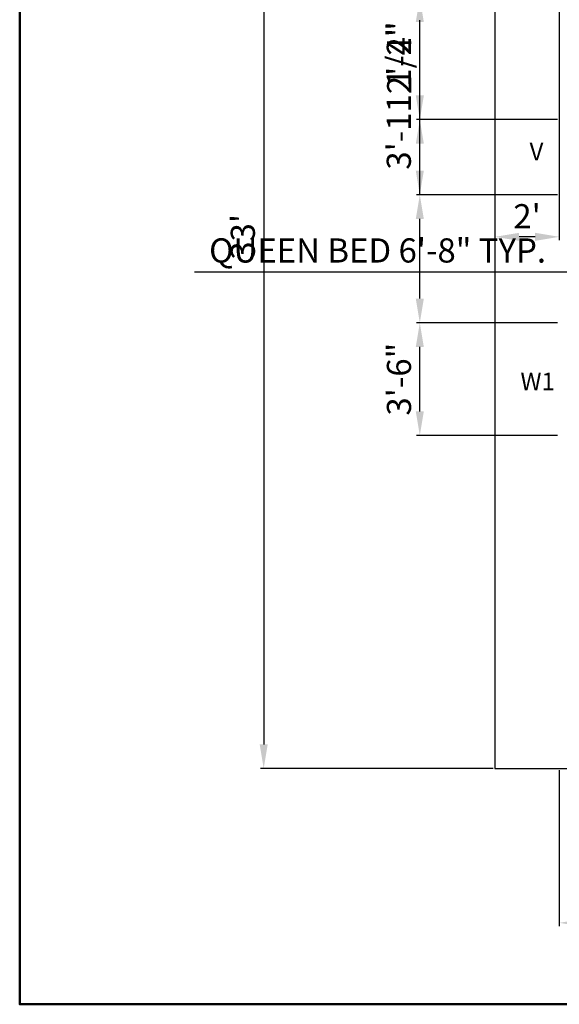
# Model space of a CAD drawing. Units: inches. Extents: x 2113 to 4530, y 1685 to 2353.
# Tile 1 of 6: x 2113 to 2314, y 1685 to 2052. Entities that reach past the tile are written whole.
import ezdxf

# ---------------------------------------------------------------- set-up
doc = ezdxf.new("R2010")
doc.units = ezdxf.units.IN
for name, color, linetype, lineweight in [('A-ANNO-DIMS', 2, 'Continuous', 18), ('A-ANNO-TEXT', 7, 'Continuous', 18), ('A-ANNO-TTLB', 7, 'Continuous', 50), ('C-PROP', 7, 'Continuous', 25), ('S-ANNO-DIMS', 2, 'Continuous', 18)]:
    doc.layers.add(name, color=color, linetype=linetype, lineweight=lineweight)
doc.styles.get("Standard").update_dxf_attribs({"font": 'arial.ttf'})
doc.dimstyles.new('ISO-25', dxfattribs={"dimtxt": 9, "dimasz": 9, "dimexe": 1.25, "dimexo": 0.625, "dimgap": 2, "dimtad": 1, "dimdec": 1, "dimlunit": 4, "dimtxsty": 'Standard', "dimcen": 2.5, "dimazin": 0, "dimtfac": 1, "dimtdec": 1, "dimtmove": 0, "dimatfit": 3, "dimfxl": 1, "dimarcsym": 0})

# ---------------------------------------------------------------- blocks, each defined once
blk = doc.blocks.new('*D8')
at = {"layer": 'A-ANNO-DIMS', "color": 0, "lineweight": -2, "transparency": 16777216}
for p, q in [((2289.11, 2168.89), (2202.39, 2168.89)), ((2203.64, 2159.89), (2203.64, 1781.89)), ((2289.11, 1772.89), (2202.39, 1772.89))]:
    blk.add_line(p, q, dxfattribs=at)
at = {"layer": 'A-ANNO-DIMS', "color": 0, "transparency": 16777216}
for points in [[(2202.14, 2159.89), (2205.14, 2159.89), (2203.64, 2168.89)], [(2202.14, 1781.89), (2205.14, 1781.89), (2203.64, 1772.89)]]:
    blk.add_solid(points, dxfattribs=at)
at = {"layer": 'Defpoints', "color": 0, "transparency": 16777216}
for p in [(2289.73, 2168.89), (2203.64, 1772.89), (2289.73, 1772.89)]:
    blk.add_point(p, dxfattribs=at)
at = {"layer": 'A-ANNO-DIMS', "color": 0, "transparency": 16777216, "insert": (2197.04, 1970.89), "char_height": 9, "attachment_point": 5, "rotation": 90}
blk.add_mtext("33'", dxfattribs=at)
blk = doc.blocks.new('*D29')
at = {"layer": 'A-ANNO-DIMS', "color": 0, "lineweight": -2, "transparency": 16777216}
for p, q in [((2289.73, 2168.26), (2289.73, 1969.64)), ((2313.73, 2150.26), (2313.73, 1969.64)), ((2304.73, 1970.89), (2298.73, 1970.89))]:
    blk.add_line(p, q, dxfattribs=at)
at = {"layer": 'A-ANNO-DIMS', "color": 0, "transparency": 16777216}
for points in [[(2298.73, 1972.39), (2298.73, 1969.39), (2289.73, 1970.89)], [(2304.73, 1972.39), (2304.73, 1969.39), (2313.73, 1970.89)]]:
    blk.add_solid(points, dxfattribs=at)
at = {"layer": 'Defpoints', "color": 0, "transparency": 16777216}
for p in [(2289.73, 2168.89), (2313.73, 2150.89), (2289.73, 1970.89)]:
    blk.add_point(p, dxfattribs=at)
at = {"layer": 'A-ANNO-DIMS', "color": 0, "transparency": 16777216, "insert": (2301.73, 1977.4), "char_height": 9, "attachment_point": 5}
blk.add_mtext("2'", dxfattribs=at)
blk = doc.blocks.new('LOT-465X396')
for p, q in [((0, 396), (0, 0)), ((0, 0), (465, 0))]:
    blk.add_line(p, q)
blk = doc.blocks.new('*D40')
at = {"layer": 'Defpoints', "color": 0, "transparency": 16777216}
for p in [(2323.25, 1957.72), (2323.25, 1945.72), (2403.25, 1945.72)]:
    blk.add_point(p, dxfattribs=at)
at = {"layer": 'S-ANNO-DIMS', "color": 0, "lineweight": -2, "transparency": 16777216}
for p, q in [((2323.25, 1946.35), (2323.25, 1958.97)), ((2403.25, 1946.35), (2403.25, 1958.97)), ((2323.25, 1957.72), (2177.86, 1957.72)), ((2394.25, 1957.72), (2332.25, 1957.72))]:
    blk.add_line(p, q, dxfattribs=at)
at = {"layer": 'S-ANNO-DIMS', "color": 0, "transparency": 16777216}
for points in [[(2332.25, 1959.22), (2332.25, 1956.22), (2323.25, 1957.72)], [(2394.25, 1959.22), (2394.25, 1956.22), (2403.25, 1957.72)]]:
    blk.add_solid(points, dxfattribs=at)
at = {"layer": 'S-ANNO-DIMS', "color": 0, "transparency": 16777216, "insert": (2246.05, 1964.65), "char_height": 9, "attachment_point": 5}
blk.add_mtext('QUEEN BED 6\'-8" TYP.', dxfattribs=at)
blk = doc.blocks.new('*D90')
at = {"layer": 'Defpoints', "color": 0, "transparency": 16777216}
for p in [(2313.73, 1772.89), (2456.73, 1772.89), (2456.73, 1715.45)]:
    blk.add_point(p, dxfattribs=at)
at = {"layer": 'S-ANNO-DIMS', "color": 0, "lineweight": -2, "transparency": 16777216}
for p, q in [((2313.73, 1772.26), (2313.73, 1714.2)), ((2456.73, 1772.26), (2456.73, 1714.2)), ((2322.73, 1715.45), (2447.73, 1715.45))]:
    blk.add_line(p, q, dxfattribs=at)
at = {"layer": 'S-ANNO-DIMS', "color": 0, "transparency": 16777216}
for points in [[(2322.73, 1716.95), (2322.73, 1713.95), (2313.73, 1715.45)], [(2447.73, 1716.95), (2447.73, 1713.95), (2456.73, 1715.45)]]:
    blk.add_solid(points, dxfattribs=at)
at = {"layer": 'S-ANNO-DIMS', "color": 0, "transparency": 16777216, "insert": (2385.23, 1721.97), "char_height": 9, "attachment_point": 5}
blk.add_mtext('11\'-11"', dxfattribs=at)
blk = doc.blocks.new('*D95')
at = {"layer": 'Defpoints', "color": 0, "transparency": 16777216}
for p in [(2261.78, 1938.89), (2313.73, 1938.89), (2313.73, 1896.89)]:
    blk.add_point(p, dxfattribs=at)
at = {"layer": 'S-ANNO-DIMS', "color": 0, "lineweight": -2, "transparency": 16777216}
for p, q in [((2313.11, 1938.89), (2260.53, 1938.89)), ((2261.78, 1905.89), (2261.78, 1929.89)), ((2313.11, 1896.89), (2260.53, 1896.89))]:
    blk.add_line(p, q, dxfattribs=at)
at = {"layer": 'S-ANNO-DIMS', "color": 0, "transparency": 16777216}
for points in [[(2260.28, 1929.89), (2263.28, 1929.89), (2261.78, 1938.89)], [(2260.28, 1905.89), (2263.28, 1905.89), (2261.78, 1896.89)]]:
    blk.add_solid(points, dxfattribs=at)
at = {"layer": 'S-ANNO-DIMS', "color": 0, "transparency": 16777216, "insert": (2255.18, 1917.89), "char_height": 9, "attachment_point": 5, "rotation": 90}
blk.add_mtext('3\'-6"', dxfattribs=at)
blk = doc.blocks.new('*D96')
at = {"layer": 'Defpoints', "color": 0, "transparency": 16777216}
for p in [(2261.78, 1986.53), (2313.73, 1986.53), (2313.73, 1938.89)]:
    blk.add_point(p, dxfattribs=at)
at = {"layer": 'S-ANNO-DIMS', "color": 0, "lineweight": -2, "transparency": 16777216}
for p, q in [((2261.78, 1986.53), (2261.78, 2051.42)), ((2313.11, 1986.53), (2260.53, 1986.53)), ((2261.78, 1947.89), (2261.78, 1977.53)), ((2313.11, 1938.89), (2260.53, 1938.89))]:
    blk.add_line(p, q, dxfattribs=at)
at = {"layer": 'S-ANNO-DIMS', "color": 0, "transparency": 16777216}
for points in [[(2260.28, 1977.53), (2263.28, 1977.53), (2261.78, 1986.53)], [(2260.28, 1947.89), (2263.28, 1947.89), (2261.78, 1938.89)]]:
    blk.add_solid(points, dxfattribs=at)
at = {"layer": 'S-ANNO-DIMS', "color": 0, "transparency": 16777216, "insert": (2255.13, 2023.47), "char_height": 9, "attachment_point": 5, "rotation": 90}
blk.add_mtext('3\'-11 1/2"', dxfattribs=at)
blk = doc.blocks.new('*D97')
at = {"layer": 'Defpoints', "color": 0, "transparency": 16777216}
for p in [(2261.78, 2014.53), (2313.73, 2014.53), (2313.73, 1986.53)]:
    blk.add_point(p, dxfattribs=at)
at = {"layer": 'S-ANNO-DIMS', "color": 0, "lineweight": -2, "transparency": 16777216}
for p, q in [((2261.78, 2014.53), (2261.78, 2051.61)), ((2313.11, 2014.53), (2260.53, 2014.53)), ((2261.78, 1995.53), (2261.78, 2005.53)), ((2313.11, 1986.53), (2260.53, 1986.53))]:
    blk.add_line(p, q, dxfattribs=at)
at = {"layer": 'S-ANNO-DIMS', "color": 0, "transparency": 16777216}
for points in [[(2260.28, 2005.53), (2263.28, 2005.53), (2261.78, 2014.53)], [(2260.28, 1995.53), (2263.28, 1995.53), (2261.78, 1986.53)]]:
    blk.add_solid(points, dxfattribs=at)
at = {"layer": 'S-ANNO-DIMS', "color": 0, "transparency": 16777216, "insert": (2255.26, 2037.57), "char_height": 9, "attachment_point": 5, "rotation": 90}
blk.add_mtext('2\'-4"', dxfattribs=at)
blk = doc.blocks.new('*D98')
at = {"layer": 'Defpoints', "color": 0, "transparency": 16777216}
for p in [(2261.78, 2059.89), (2313.73, 2059.89), (2313.73, 2014.53)]:
    blk.add_point(p, dxfattribs=at)
at = {"layer": 'S-ANNO-DIMS', "color": 0, "lineweight": -2, "transparency": 16777216}
for p, q in [((2261.78, 2059.89), (2261.78, 2117.78)), ((2313.11, 2059.89), (2260.53, 2059.89)), ((2261.78, 2023.53), (2261.78, 2050.89)), ((2313.11, 2014.53), (2260.53, 2014.53))]:
    blk.add_line(p, q, dxfattribs=at)
at = {"layer": 'S-ANNO-DIMS', "color": 0, "transparency": 16777216}
for points in [[(2260.28, 2050.89), (2263.28, 2050.89), (2261.78, 2059.89)], [(2260.28, 2023.53), (2263.28, 2023.53), (2261.78, 2014.53)]]:
    blk.add_solid(points, dxfattribs=at)
at = {"layer": 'S-ANNO-DIMS', "color": 0, "transparency": 16777216, "insert": (2255.13, 2093.33), "char_height": 9, "attachment_point": 5, "rotation": 90}
blk.add_mtext('3\'-9 1/2"', dxfattribs=at)

msp = doc.modelspace()

# ---------------------------------------------------------------- linework, layer by layer
at = {"layer": 'A-ANNO-TTLB'}
msp.add_lwpolyline([(2112.77, 2352.97), (4498.42, 2352.97), (4498.42, 1685.12), (2112.77, 1685.12)], close=True, dxfattribs=at)

# ---------------------------------------------------------------- block references
at = {"layer": 'C-PROP'}
msp.add_blockref('LOT-465X396', (2289.73, 1772.89), dxfattribs=at)

# ---------------------------------------------------------------- texts
at = {"layer": 'A-ANNO-TEXT'}
for s, p in [('V', (2302.66, 1999.4)), ('W1', (2299.26, 1913.77))]:
    msp.add_text(s, height=6.54, dxfattribs=at).set_placement(p)

# ---------------------------------------------------------------- dimensions: what is measured, and where the dimension line sits
at = {"layer": 'A-ANNO-DIMS'}
dim = msp.add_linear_dim(base=(2203.64, 1772.89), p1=(2289.73, 2168.89), p2=(2289.73, 1772.89), angle=90, dimstyle='ISO-25', override={"dimclrd": 0, "dimclre": 0, "dimclrt": 0}, dxfattribs=at)
dim.commit()
dim.dimension.update_dxf_attribs({"geometry": '*D8', "text_midpoint": (2197.04, 1970.89)})
dim = msp.add_linear_dim(base=(2289.73, 1970.89), p1=(2313.73, 2150.89), p2=(2289.73, 2168.89), dimstyle='ISO-25', override={"dimclrd": 0, "dimclre": 0, "dimclrt": 0}, dxfattribs=at)
dim.commit()
dim.dimension.update_dxf_attribs({"geometry": '*D29', "text_midpoint": (2301.73, 1977.4)})
at = {"layer": 'S-ANNO-DIMS'}
for base, p1, p2, picture, middle in [((2261.78, 2059.89), (2313.73, 2014.53), (2313.73, 2059.89), '*D98', (2255.13, 2093.33)), ((2261.78, 1986.53), (2313.73, 1938.89), (2313.73, 1986.53), '*D96', (2255.13, 2023.47)), ((2261.78, 2014.53), (2313.73, 1986.53), (2313.73, 2014.53), '*D97', (2255.26, 2037.57)), ((2261.78, 1938.89), (2313.73, 1896.89), (2313.73, 1938.89), '*D95', (2255.18, 1917.89))]:
    dim = msp.add_linear_dim(base=base, p1=p1, p2=p2, angle=90, dimstyle='ISO-25', override={"dimdec": 1, "dimlfac": 1, "dimrnd": 0, "dimzin": 1, "dimdsep": 46, "dimlunit": 4, "dimfrac": 2}, dxfattribs=at)
    dim.commit()
    dim.dimension.update_dxf_attribs({"geometry": picture, "text_midpoint": middle})
dim = msp.add_linear_dim(base=(2323.25, 1957.72), p1=(2403.25, 1945.72), p2=(2323.25, 1945.72), angle=180, text='QUEEN BED <> TYP.', dimstyle='ISO-25', override={"dimdec": 1, "dimlfac": 1, "dimrnd": 0, "dimzin": 1, "dimdsep": 46, "dimlunit": 4, "dimfrac": 2}, dxfattribs=at)
dim.commit()
dim.dimension.update_dxf_attribs({"geometry": '*D40', "text_midpoint": (2246.05, 1964.65)})
dim = msp.add_linear_dim(base=(2456.73, 1715.45), p1=(2313.73, 1772.89), p2=(2456.73, 1772.89), dimstyle='ISO-25', override={"dimdec": 1, "dimlfac": 1, "dimrnd": 0, "dimzin": 1, "dimdsep": 46, "dimlunit": 4, "dimfrac": 2}, dxfattribs=at)
dim.commit()
dim.dimension.update_dxf_attribs({"geometry": '*D90', "text_midpoint": (2385.23, 1721.97)})

doc.saveas('drawing.dxf')
